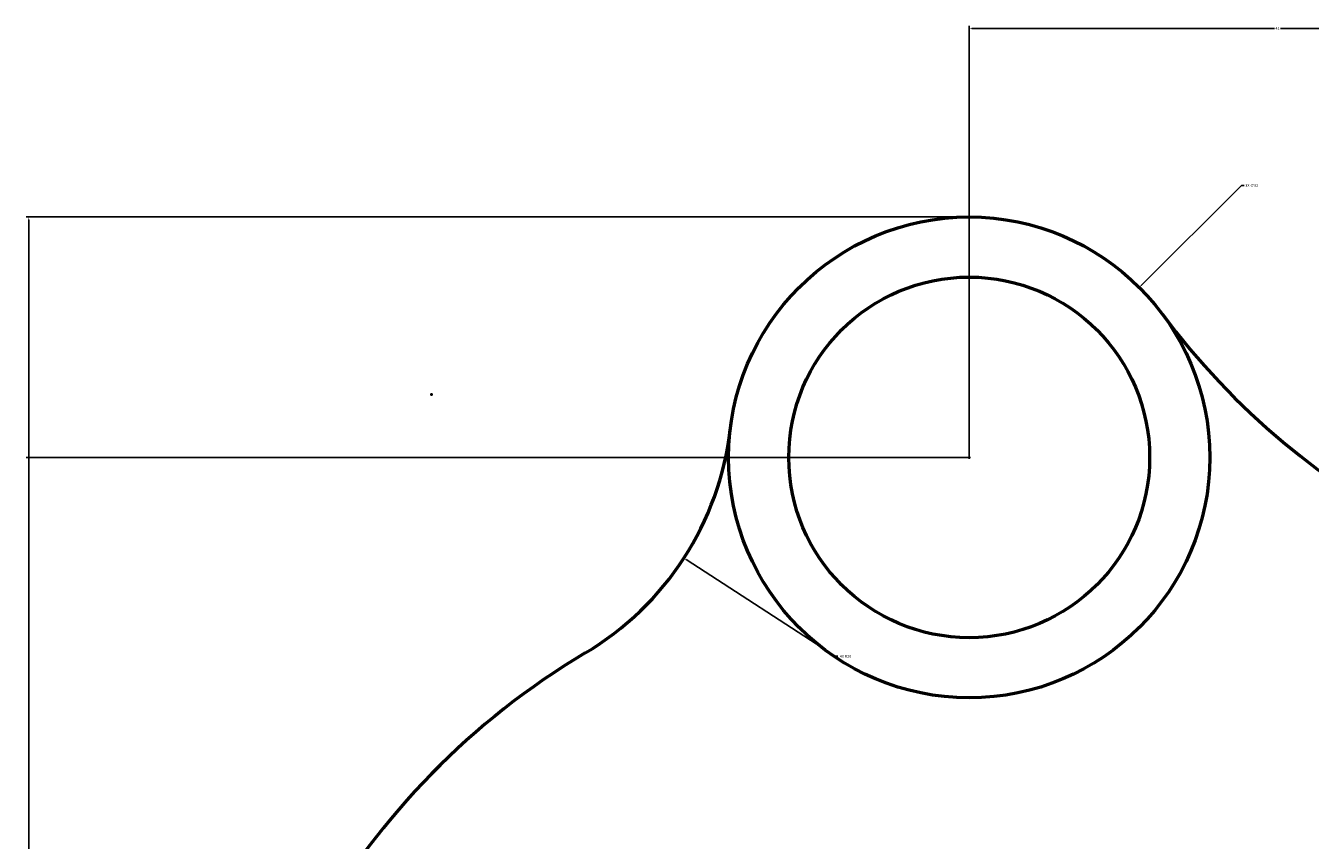
# Model space of a CAD drawing. Units: inches. Extents: x -307 to -76, y 16 to 196.
# Tile 3 of 7: x -307 to -222, y 132 to 186. Entities that reach past the tile are written whole.
import ezdxf

# ---------------------------------------------------------------- set-up
doc = ezdxf.new("R2010")
doc.units = ezdxf.units.IN
doc.header["$MEASUREMENT"] = 0
doc.layers.add('M-DIMS', color=2, linetype='Continuous', lineweight=18)
doc.layers.add('M-OUTL', color=7, linetype='Continuous', lineweight=50)
doc.styles.get("Standard").update_dxf_attribs({"font": 'arial.ttf'})
doc.dimstyles.get("Standard").update_dxf_attribs({"dimtxt": 0.18, "dimasz": 0.18, "dimexe": 0.18, "dimexo": 0.0625, "dimgap": 0.09, "dimtad": 0, "dimtih": 1, "dimtoh": 1, "dimdec": 4, "dimzin": 0, "dimdsep": 46, "dimtxsty": 'Standard', "dimcen": 0.09, "dimadec": 0, "dimazin": 0, "dimtfac": 1, "dimtdec": 4, "dimtofl": 0, "dimtmove": 0, "dimatfit": 3, "dimfxl": 1, "dimtolj": 1, "dimtzin": 0, "dimarcsym": 0})

# ---------------------------------------------------------------- blocks, each defined once
blk = doc.blocks.new('BORE-D24-RIM-D32')
for radius in [16, 12]:
    blk.add_circle((16, 16), radius)
blk = doc.blocks.new('*D3')
at = {"layer": 'Defpoints', "color": 0, "transparency": 16777216}
for p in [(-306.94, 173), (-244.39, 173), (-244.39, 29)]:
    blk.add_point(p, dxfattribs=at)
at = {"layer": 'M-DIMS', "color": 0, "lineweight": -2, "transparency": 16777216}
for p, q in [((-244.452, 173), (-307.12, 173)), ((-306.94, 172.82), (-306.94, 101.18)), ((-306.94, 29.18), (-306.94, 100.82)), ((-244.452, 29), (-307.12, 29))]:
    blk.add_line(p, q, dxfattribs=at)
at = {"layer": 'M-DIMS', "color": 0, "transparency": 16777216}
for points in [[(-306.97, 172.82), (-306.91, 172.82), (-306.94, 173)], [(-306.97, 29.18), (-306.91, 29.18), (-306.94, 29)]]:
    blk.add_solid(points, dxfattribs=at)
at = {"layer": 'M-DIMS', "color": 0, "transparency": 16777216, "insert": (-306.94, 101), "char_height": 0.18, "attachment_point": 5}
blk.add_mtext('\\A1;144', dxfattribs=at)
blk = doc.blocks.new('*D4')
at = {"layer": 'Defpoints', "color": 0, "transparency": 16777216}
for p in [(-203.39, 185.55), (-244.39, 157), (-203.39, 101)]:
    blk.add_point(p, dxfattribs=at)
at = {"layer": 'M-DIMS', "color": 0, "lineweight": -2, "transparency": 16777216}
for p, q in [((-244.39, 157.062), (-244.39, 185.73)), ((-244.21, 185.55), (-224.095, 185.55)), ((-203.57, 185.55), (-223.684, 185.55)), ((-203.39, 101.062), (-203.39, 185.73))]:
    blk.add_line(p, q, dxfattribs=at)
at = {"layer": 'M-DIMS', "color": 0, "transparency": 16777216}
for points in [[(-244.21, 185.58), (-244.21, 185.52), (-244.39, 185.55)], [(-203.57, 185.58), (-203.57, 185.52), (-203.39, 185.55)]]:
    blk.add_solid(points, dxfattribs=at)
at = {"layer": 'M-DIMS', "color": 0, "transparency": 16777216, "insert": (-223.89, 185.55), "char_height": 0.18, "attachment_point": 5}
blk.add_mtext('\\A1;41', dxfattribs=at)
blk = doc.blocks.new('*D7')
at = {"layer": 'Defpoints', "color": 0, "transparency": 16777216}
for p in [(-306.94, 157), (-244.39, 157), (-244.39, 101)]:
    blk.add_point(p, dxfattribs=at)
at = {"layer": 'M-DIMS', "color": 0, "lineweight": -2, "transparency": 16777216}
for p, q in [((-244.452, 157), (-307.12, 157)), ((-306.94, 156.82), (-306.94, 129.182)), ((-306.94, 101.18), (-306.94, 128.818)), ((-244.452, 101), (-307.12, 101))]:
    blk.add_line(p, q, dxfattribs=at)
at = {"layer": 'M-DIMS', "color": 0, "transparency": 16777216}
for points in [[(-306.97, 156.82), (-306.91, 156.82), (-306.94, 157)], [(-306.97, 101.18), (-306.91, 101.18), (-306.94, 101)]]:
    blk.add_solid(points, dxfattribs=at)
at = {"layer": 'M-DIMS', "color": 0, "transparency": 16777216, "insert": (-306.94, 129), "char_height": 0.18, "attachment_point": 5}
blk.add_mtext('\\A1;56', dxfattribs=at)
blk = doc.blocks.new('*D11')
at = {"layer": 'Defpoints', "color": 0, "transparency": 16777216}
for p in [(-280.146, 161.179), (-263.368, 150.293)]:
    blk.add_point(p, dxfattribs=at)
at = {"layer": 'M-DIMS', "color": 0, "lineweight": -2, "transparency": 16777216}
for p, q in [((-280.236, 161.179), (-280.056, 161.179)), ((-280.146, 161.089), (-280.146, 161.269)), ((-253.301, 143.762), (-263.217, 150.195)), ((-253.121, 143.762), (-253.301, 143.762))]:
    blk.add_line(p, q, dxfattribs=at)
at = {"layer": 'M-DIMS', "color": 0, "transparency": 16777216}
blk.add_solid([(-263.201, 150.22), (-263.233, 150.17), (-263.368, 150.293)], dxfattribs=at)
at = {"layer": 'M-DIMS', "color": 0, "transparency": 16777216, "insert": (-252.62, 143.762), "char_height": 0.18, "attachment_point": 5}
blk.add_mtext('\\A1;4X R20', dxfattribs=at)
blk = doc.blocks.new('*D20')
at = {"layer": 'Defpoints', "color": 0, "transparency": 16777216}
for p in [(-233.076, 168.314), (-255.703, 145.686)]:
    blk.add_point(p, dxfattribs=at)
at = {"layer": 'M-DIMS', "color": 0, "lineweight": -2, "transparency": 16777216}
for p, q in [((-226.288, 175.102), (-232.949, 168.441)), ((-226.108, 175.102), (-226.288, 175.102)), ((-244.48, 157), (-244.3, 157)), ((-244.39, 156.91), (-244.39, 157.09))]:
    blk.add_line(p, q, dxfattribs=at)
at = {"layer": 'M-DIMS', "color": 0, "transparency": 16777216}
blk.add_solid([(-232.97, 168.462), (-232.928, 168.42), (-233.076, 168.314)], dxfattribs=at)
at = {"layer": 'M-DIMS', "color": 0, "transparency": 16777216, "insert": (-225.604, 175.102), "char_height": 0.18, "attachment_point": 5}
blk.add_mtext('\\A1;3X ∅32', dxfattribs=at)

msp = doc.modelspace()

# ---------------------------------------------------------------- linework, layer by layer
at = {"layer": 'M-OUTL'}
for centre, radius, start, end in [((-191.39, 196.332), 50, 216.57954, 323.42046), ((-280.146, 161.179), 20, 300.71777, 353.33457), ((-244.39, 101), 50, 120.71777, 239.28223)]:
    msp.add_arc(centre, radius, start, end, dxfattribs=at)

# ---------------------------------------------------------------- block references
msp.add_blockref('BORE-D24-RIM-D32', (-260.39, 141), dxfattribs=at)

# ---------------------------------------------------------------- dimensions: what is measured, and where the dimension line sits
at = {"layer": 'M-DIMS'}
dim = msp.add_linear_dim(base=(-203.39, 185.55), p1=(-244.39, 157), p2=(-203.39, 101), dimstyle='Standard', override={"dimdec": 0, "dimlfac": 1, "dimrnd": 0, "dimzin": 0, "dimdsep": 46, "dimlunit": 2}, dxfattribs=at)
dim.commit()
dim.dimension.update_dxf_attribs({"geometry": '*D4', "text_midpoint": (-223.89, 185.55)})
dim = msp.add_diameter_dim_2p(p1=(-255.703, 145.686), p2=(-233.076, 168.314), text='3X <>', dimstyle='Standard', override={"dimdec": 0, "dimlfac": 1, "dimrnd": 0, "dimzin": 0, "dimdsep": 46, "dimlunit": 2}, dxfattribs=at)
dim.commit()
dim.dimension.update_dxf_attribs({"geometry": '*D20', "text_midpoint": (-225.604, 175.102), "dimtype": 163})
for base, p1, p2, picture, middle in [((-306.94, 173), (-244.39, 29), (-244.39, 173), '*D3', (-306.94, 101)), ((-306.94, 157), (-244.39, 101), (-244.39, 157), '*D7', (-306.94, 129))]:
    dim = msp.add_linear_dim(base=base, p1=p1, p2=p2, angle=90, dimstyle='Standard', override={"dimdec": 0, "dimlfac": 1, "dimrnd": 0, "dimzin": 0, "dimdsep": 46, "dimlunit": 2}, dxfattribs=at)
    dim.commit()
    dim.dimension.update_dxf_attribs({"geometry": picture, "text_midpoint": middle})
dim = msp.add_radius_dim(center=(-280.146, 161.179), mpoint=(-263.368, 150.293), text='4X <>', dimstyle='Standard', override={"dimdec": 0, "dimlfac": 1, "dimrnd": 0, "dimzin": 0, "dimdsep": 46, "dimlunit": 2}, dxfattribs=at)
dim.commit()
dim.dimension.update_dxf_attribs({"geometry": '*D11', "text_midpoint": (-252.62, 143.762), "dimtype": 164})

doc.saveas('drawing.dxf')
